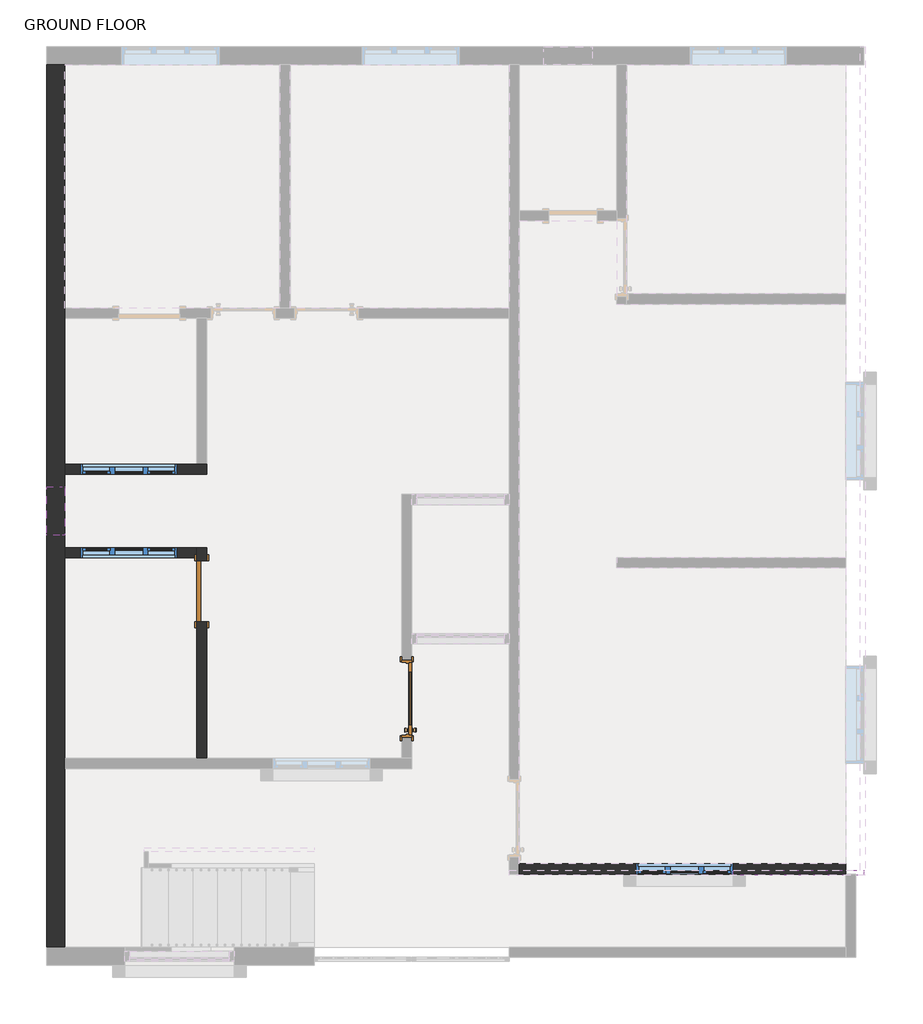
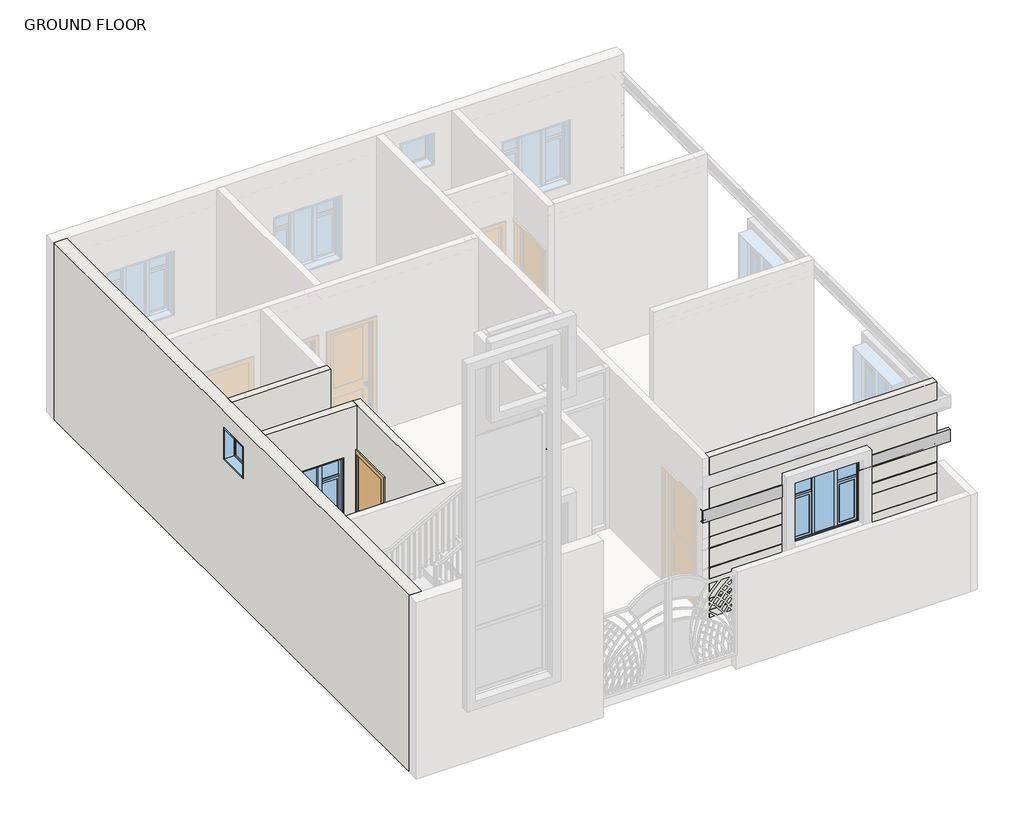
# One storey, part 2 of 7: 5 walls, 4 windows, 2 doors, 1 proxy.
# Revit data of these elements (continued)
# Element 4 (IfcWall) (continued)
#   Materials on its faces: "OUTER WALL"
# Element 5 (IfcWall, "INNER WALL 5\"")
#   built-in parameter 1001111 = -1' - 0"
#   Top Offset = 0' - 0"
#   Base Offset = -1' - 0"
#   wall height = 11' - 0"
#   Phase Created = New Construction
#   Base Constraint = GROUND FLOOR
#   Top Constraint = FIRST FLOOR
#   Materials on its faces: "OUTER WALL"
# Elements 6, 7, 8 (IfcWall, "INNER WALL 5\"")
#   Top Offset = 0' - 0"
#   Base Offset = 0' - 0"
#   wall height = 10' - 0"
#   Phase Created = New Construction
#   Base Constraint = GROUND FLOOR
#   Top Constraint = FIRST FLOOR
#   Materials on its faces: "OUTER WALL"
# Element 9 (IfcWindow, "Fixed : opening window 2' x 2'")
#   Mark = "1"
#   Phase Created = New Construction
#   Materials on its faces: "Sash", "Glass"
# Element 10 (IfcWindow, "Window-Casement-Triple-Side-Transom : window 4' x 4'")
#   Mark = "8"
#   Window Inset = 0' - 0 5/8"
#   Frame Gap 3 = 0' - 1 83/128"
#   Frame Gap 2 = 0' - 0 5/8"
#   Phase Created = New Construction
#   Materials on its faces: "Metal - Aluminum", "Glass"
# Element 11 (IfcWindow, "Window-Casement-Triple-Side-Transom : window 4' x 4'")
#   Mark = "12"
#   Window Inset = 0' - 0 5/8"
#   Frame Gap 3 = 0' - 1 83/128"
#   Frame Gap 2 = 0' - 0 5/8"
#   Phase Created = New Construction
#   Materials on its faces: "Metal - Aluminum", "Glass"
# Element 12 (IfcWindow, "Window-Casement-Triple-Side-Transom : window 4' x 4'")
#   Mark = "13"
#   Window Inset = 0' - 0 5/8"
#   Frame Gap 3 = 0' - 1 83/128"
#   Frame Gap 2 = 0' - 0 5/8"
#   Phase Created = New Construction
#   Materials on its faces: "Metal - Aluminum", "Glass"
# Materials
#   "Cherry": class "Wood", colour RGB 226 177 128, transparency 0, Description = "Prunus Serotina", Cost = 0
#   "Aluminum": class "Metal", colour RGB 247 247 247, transparency 0, Description = "Aluminum 6061", Cost = 0
#   "Door - Panel": class "Wood", colour RGB 210 159 95, transparency 0, Cost = 0
#   "Door - Frame": colour RGB 118 70 51, transparency 0, Cost = 0
#   "OUTER WALL": class "Generic", colour RGB 245 245 240, transparency 0, Cost = 0
#   "Glass": class "Glass", colour RGB 0 128 192, transparency 0.75, Description = "Soda Lime Glass", Cost = 0
#   "Sash": class "Wood", colour RGB 224 178 126, transparency 0, Cost = 0
#   "Metal - Aluminum": class "Metal", colour RGB 247 247 247, transparency 0
